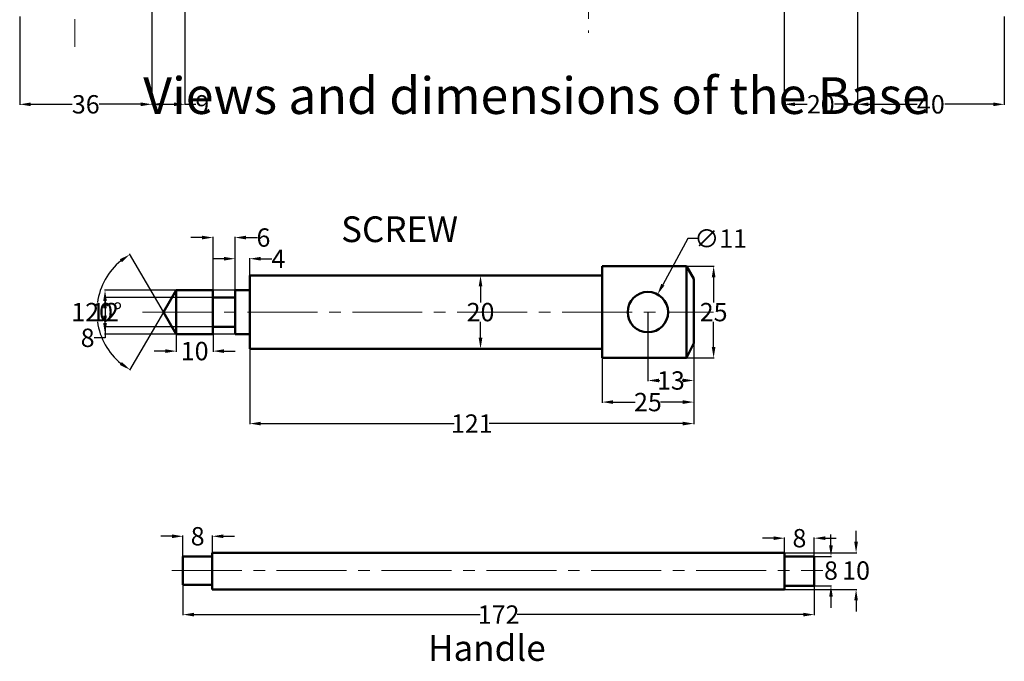
# Model space of a CAD drawing. Units: metres. Extents: x -2793 to -2360, y -31 to 491.
# Tile 1 of 4: x -2760 to -2492, y -31 to 144. Entities that reach past the tile are written whole.
import ezdxf

# ---------------------------------------------------------------- set-up
doc = ezdxf.new("R2010")
doc.units = ezdxf.units.M
doc.linetypes.add('CENTER2', pattern=[28.575, 19.05, -3.175, 3.175, -3.175])
for name, color, linetype, lineweight in [('M-CNTR', 9, 'CENTER2', 18), ('M-DIMS', 2, 'Continuous', 25), ('M-OUTL', 7, 'Continuous', 50), ('M-TEXT', 7, 'Continuous', 25)]:
    doc.layers.add(name, color=color, linetype=linetype, lineweight=lineweight)
doc.styles.get("Standard").update_dxf_attribs({"font": 'arial.ttf'})
doc.dimstyles.get("Standard").update_dxf_attribs({"dimtxt": 5, "dimasz": 3, "dimexe": 0.18, "dimexo": 0.0625, "dimgap": 0.09, "dimtad": 0, "dimtih": 1, "dimtoh": 1, "dimdec": 0, "dimzin": 0, "dimdsep": 46, "dimtxsty": 'Standard', "dimcen": 0.09, "dimclrd": 254, "dimclre": 254, "dimadec": 0, "dimazin": 0, "dimtfac": 1, "dimtdec": 0, "dimtofl": 0, "dimtmove": 0, "dimatfit": 3, "dimfxl": 1, "dimtolj": 1, "dimtzin": 0, "dimarcsym": 0})

# ---------------------------------------------------------------- blocks, each defined once
blk = doc.blocks.new('*D33')
at = {"layer": 'Defpoints', "color": 0, "transparency": 16777216}
for p in [(-2543.38, -1.94), (-2543.38, -9.94), (-2538.83, -9.94)]:
    blk.add_point(p, dxfattribs=at)
at = {"layer": 'M-DIMS', "color": 0, "lineweight": -2, "transparency": 16777216}
for p, q in [((-2538.83, 1.06), (-2538.83, 4.06)), ((-2543.32, -1.94), (-2538.65, -1.94)), ((-2543.32, -9.94), (-2538.65, -9.94)), ((-2538.83, -12.94), (-2538.83, -15.94))]:
    blk.add_line(p, q, dxfattribs=at)
at = {"layer": 'M-DIMS', "color": 0, "transparency": 16777216}
for points in [[(-2539.33, 1.06), (-2538.33, 1.06), (-2538.83, -1.94)], [(-2539.33, -12.94), (-2538.33, -12.94), (-2538.83, -9.94)]]:
    blk.add_solid(points, dxfattribs=at)
at = {"layer": 'M-DIMS', "color": 0, "transparency": 16777216, "insert": (-2538.83, -5.8), "char_height": 5, "attachment_point": 5}
blk.add_mtext('\\A1;{\\fTimes New Roman|b0|i0|c0|p18;8}', dxfattribs=at)
blk = doc.blocks.new('*D34')
at = {"layer": 'Defpoints', "color": 0, "transparency": 16777216}
for p in [(-2707.38, 3.55), (-2715.38, -1.94), (-2707.38, -1.94)]:
    blk.add_point(p, dxfattribs=at)
at = {"layer": 'M-DIMS', "color": 0, "lineweight": -2, "transparency": 16777216}
for p, q in [((-2718.38, 3.55), (-2721.38, 3.55)), ((-2715.38, -1.88), (-2715.38, 3.73)), ((-2707.38, -1.88), (-2707.38, 3.73)), ((-2704.38, 3.55), (-2701.38, 3.55))]:
    blk.add_line(p, q, dxfattribs=at)
at = {"layer": 'M-DIMS', "color": 0, "transparency": 16777216}
for points in [[(-2718.38, 4.05), (-2718.38, 3.05), (-2715.38, 3.55)], [(-2704.38, 4.05), (-2704.38, 3.05), (-2707.38, 3.55)]]:
    blk.add_solid(points, dxfattribs=at)
at = {"layer": 'M-DIMS', "color": 0, "transparency": 16777216, "insert": (-2711.38, 3.55), "char_height": 5, "attachment_point": 5}
blk.add_mtext('\\A1;{\\fTimes New Roman|b0|i0|c0|p18;8}', dxfattribs=at)
blk = doc.blocks.new('*D35')
at = {"layer": 'Defpoints', "color": 0, "transparency": 16777216}
for p in [(-2551.48, 3.03), (-2551.48, -1.94), (-2543.38, -1.94)]:
    blk.add_point(p, dxfattribs=at)
at = {"layer": 'M-DIMS', "color": 0, "lineweight": -2, "transparency": 16777216}
for p, q in [((-2554.48, 3.03), (-2557.48, 3.03)), ((-2551.48, -1.88), (-2551.48, 3.21)), ((-2543.38, -1.88), (-2543.38, 3.21)), ((-2540.38, 3.03), (-2537.38, 3.03))]:
    blk.add_line(p, q, dxfattribs=at)
at = {"layer": 'M-DIMS', "color": 0, "transparency": 16777216}
for points in [[(-2554.48, 3.53), (-2554.48, 2.53), (-2551.48, 3.03)], [(-2540.38, 3.53), (-2540.38, 2.53), (-2543.38, 3.03)]]:
    blk.add_solid(points, dxfattribs=at)
at = {"layer": 'M-DIMS', "color": 0, "transparency": 16777216, "insert": (-2547.43, 3.03), "char_height": 5, "attachment_point": 5}
blk.add_mtext('\\A1;{\\fTimes New Roman|b0|i0|c0|p18;8}', dxfattribs=at)
blk = doc.blocks.new('*D36')
at = {"layer": 'Defpoints', "color": 0, "transparency": 16777216}
for p in [(-2715.38, -9.66), (-2543.38, -9.94), (-2715.38, -17.79)]:
    blk.add_point(p, dxfattribs=at)
at = {"layer": 'M-DIMS', "color": 0, "lineweight": -2, "transparency": 16777216}
for p, q in [((-2715.38, -9.73), (-2715.38, -17.97)), ((-2543.38, -10), (-2543.38, -17.97)), ((-2712.38, -17.79), (-2634.43, -17.79)), ((-2546.38, -17.79), (-2624.34, -17.79))]:
    blk.add_line(p, q, dxfattribs=at)
at = {"layer": 'M-DIMS', "color": 0, "transparency": 16777216}
for points in [[(-2712.38, -17.29), (-2712.38, -18.29), (-2715.38, -17.79)], [(-2546.38, -17.29), (-2546.38, -18.29), (-2543.38, -17.79)]]:
    blk.add_solid(points, dxfattribs=at)
at = {"layer": 'M-DIMS', "color": 0, "transparency": 16777216, "insert": (-2629.38, -17.79), "char_height": 5, "attachment_point": 5}
blk.add_mtext('\\A1;{\\fTimes New Roman|b0|i0|c0|p18;172}', dxfattribs=at)
blk = doc.blocks.new('*D37')
at = {"layer": 'Defpoints', "color": 0, "transparency": 16777216}
for p in [(-2551.48, -0.94), (-2551.48, -10.94), (-2531.99, -10.94)]:
    blk.add_point(p, dxfattribs=at)
at = {"layer": 'M-DIMS', "color": 0, "lineweight": -2, "transparency": 16777216}
for p, q in [((-2531.99, 2.06), (-2531.99, 5.06)), ((-2551.42, -0.94), (-2531.81, -0.94)), ((-2551.42, -10.94), (-2531.81, -10.94)), ((-2531.99, -13.94), (-2531.99, -16.94))]:
    blk.add_line(p, q, dxfattribs=at)
at = {"layer": 'M-DIMS', "color": 0, "transparency": 16777216}
for points in [[(-2532.49, 2.06), (-2531.49, 2.06), (-2531.99, -0.94)], [(-2532.49, -13.94), (-2531.49, -13.94), (-2531.99, -10.94)]]:
    blk.add_solid(points, dxfattribs=at)
at = {"layer": 'M-DIMS', "color": 0, "transparency": 16777216, "insert": (-2531.99, -5.79), "char_height": 5, "attachment_point": 5}
blk.add_mtext('\\A1;{\\fTimes New Roman|b0|i0|c0|p18;10}', dxfattribs=at)
blk = doc.blocks.new('*D38')
at = {"layer": 'Defpoints', "color": 0, "transparency": 16777216}
for p in [(-2697.2, 54.62), (-2576.2, 56.14), (-2576.2, 34.25)]:
    blk.add_point(p, dxfattribs=at)
at = {"layer": 'M-DIMS', "color": 0, "lineweight": -2, "transparency": 16777216}
for p, q in [((-2697.2, 54.56), (-2697.2, 34.07)), ((-2576.2, 56.08), (-2576.2, 34.07)), ((-2694.2, 34.25), (-2641.45, 34.25)), ((-2579.2, 34.25), (-2631.96, 34.25))]:
    blk.add_line(p, q, dxfattribs=at)
at = {"layer": 'M-DIMS', "color": 0, "transparency": 16777216}
for points in [[(-2694.2, 34.75), (-2694.2, 33.75), (-2697.2, 34.25)], [(-2579.2, 34.75), (-2579.2, 33.75), (-2576.2, 34.25)]]:
    blk.add_solid(points, dxfattribs=at)
at = {"layer": 'M-DIMS', "color": 0, "transparency": 16777216, "insert": (-2636.7, 34.25), "char_height": 5, "attachment_point": 5}
blk.add_mtext('\\A1;{\\fTimes New Roman|b0|i0|c0|p18;121}', dxfattribs=at)
blk = doc.blocks.new('*D39')
at = {"layer": 'Defpoints', "color": 0, "transparency": 16777216}
for p in [(-2630.64, 74.62), (-2634.31, 54.62), (-2630.64, 54.62)]:
    blk.add_point(p, dxfattribs=at)
at = {"layer": 'M-DIMS', "color": 0, "lineweight": -2, "transparency": 16777216}
for p, q in [((-2630.71, 74.62), (-2634.49, 74.62)), ((-2634.31, 71.62), (-2634.31, 67.26)), ((-2634.31, 57.62), (-2634.31, 61.99)), ((-2630.71, 54.62), (-2634.49, 54.62))]:
    blk.add_line(p, q, dxfattribs=at)
at = {"layer": 'M-DIMS', "color": 0, "transparency": 16777216}
for points in [[(-2634.81, 71.62), (-2633.81, 71.62), (-2634.31, 74.62)], [(-2634.81, 57.62), (-2633.81, 57.62), (-2634.31, 54.62)]]:
    blk.add_solid(points, dxfattribs=at)
at = {"layer": 'M-DIMS', "color": 0, "transparency": 16777216, "insert": (-2634.31, 64.62), "char_height": 5, "attachment_point": 5}
blk.add_mtext('\\A1;{\\fTimes New Roman|b0|i0|c0|p18;20}', dxfattribs=at)
blk = doc.blocks.new('*D40')
at = {"layer": 'Defpoints', "color": 0, "transparency": 16777216}
for p in [(-2601.2, 52.12), (-2576.2, 52.12), (-2576.2, 40.11)]:
    blk.add_point(p, dxfattribs=at)
at = {"layer": 'M-DIMS', "color": 0, "lineweight": -2, "transparency": 16777216}
for p, q in [((-2601.2, 52.06), (-2601.2, 39.93)), ((-2576.2, 52.06), (-2576.2, 39.93)), ((-2598.2, 40.11), (-2592.16, 40.11)), ((-2579.2, 40.11), (-2585.25, 40.11))]:
    blk.add_line(p, q, dxfattribs=at)
at = {"layer": 'M-DIMS', "color": 0, "transparency": 16777216}
for points in [[(-2598.2, 40.61), (-2598.2, 39.61), (-2601.2, 40.11)], [(-2579.2, 40.61), (-2579.2, 39.61), (-2576.2, 40.11)]]:
    blk.add_solid(points, dxfattribs=at)
at = {"layer": 'M-DIMS', "color": 0, "transparency": 16777216, "insert": (-2588.7, 40.11), "char_height": 5, "attachment_point": 5}
blk.add_mtext('\\A1;{\\fTimes New Roman|b0|i0|c0|p18;25}', dxfattribs=at)
blk = doc.blocks.new('*D41')
at = {"layer": 'Defpoints', "color": 0, "transparency": 16777216}
for p in [(-2588.7, 64.62), (-2576.2, 64.62), (-2576.2, 45.99)]:
    blk.add_point(p, dxfattribs=at)
at = {"layer": 'M-DIMS', "color": 0, "lineweight": -2, "transparency": 16777216}
for p, q in [((-2588.7, 64.56), (-2588.7, 45.81)), ((-2576.2, 64.56), (-2576.2, 45.81)), ((-2585.7, 45.99), (-2585.5, 45.99)), ((-2579.2, 45.99), (-2579.41, 45.99))]:
    blk.add_line(p, q, dxfattribs=at)
at = {"layer": 'M-DIMS', "color": 0, "transparency": 16777216}
for points in [[(-2585.7, 46.49), (-2585.7, 45.49), (-2588.7, 45.99)], [(-2579.2, 46.49), (-2579.2, 45.49), (-2576.2, 45.99)]]:
    blk.add_solid(points, dxfattribs=at)
at = {"layer": 'M-DIMS', "color": 0, "transparency": 16777216, "insert": (-2582.45, 45.99), "char_height": 5, "attachment_point": 5}
blk.add_mtext('\\A1;{\\fTimes New Roman|b0|i0|c0|p18;13}', dxfattribs=at)
blk = doc.blocks.new('*D42')
at = {"layer": 'Defpoints', "color": 0, "transparency": 16777216}
for p in [(-2578.2, 77.12), (-2578.2, 52.12), (-2570.8, 52.12)]:
    blk.add_point(p, dxfattribs=at)
at = {"layer": 'M-DIMS', "color": 0, "lineweight": -2, "transparency": 16777216}
for p, q in [((-2578.14, 77.12), (-2570.62, 77.12)), ((-2570.8, 74.12), (-2570.8, 67.26)), ((-2570.8, 55.12), (-2570.8, 61.99)), ((-2578.14, 52.12), (-2570.62, 52.12))]:
    blk.add_line(p, q, dxfattribs=at)
at = {"layer": 'M-DIMS', "color": 0, "transparency": 16777216}
for points in [[(-2571.3, 74.12), (-2570.3, 74.12), (-2570.8, 77.12)], [(-2571.3, 55.12), (-2570.3, 55.12), (-2570.8, 52.12)]]:
    blk.add_solid(points, dxfattribs=at)
at = {"layer": 'M-DIMS', "color": 0, "transparency": 16777216, "insert": (-2570.8, 64.62), "char_height": 5, "attachment_point": 5}
blk.add_mtext('\\A1;{\\fTimes New Roman|b0|i0|c0|p18;25}', dxfattribs=at)
blk = doc.blocks.new('*D43')
at = {"layer": 'Defpoints', "color": 0, "transparency": 16777216}
for p in [(-2586.08, 69.45), (-2591.33, 59.79)]:
    blk.add_point(p, dxfattribs=at)
at = {"layer": 'M-DIMS', "color": 0, "lineweight": -2, "transparency": 16777216}
for p, q in [((-2577.81, 84.65), (-2584.64, 72.09)), ((-2574.77, 84.65), (-2577.81, 84.65)), ((-2588.79, 64.62), (-2588.61, 64.62)), ((-2588.7, 64.53), (-2588.7, 64.71))]:
    blk.add_line(p, q, dxfattribs=at)
at = {"layer": 'M-DIMS', "color": 0, "transparency": 16777216}
blk.add_solid([(-2585.08, 72.33), (-2584.2, 71.85), (-2586.08, 69.45)], dxfattribs=at)
at = {"layer": 'M-DIMS', "color": 0, "transparency": 16777216, "insert": (-2568.9, 84.65), "char_height": 5, "attachment_point": 5}
blk.add_mtext('\\A1;{\\fTimes New Roman|b0|i0|c0|p18;∅11}', dxfattribs=at)
blk = doc.blocks.new('*D44')
at = {"layer": 'Defpoints', "color": 0, "transparency": 16777216}
for p in [(-2697.2, 79.16), (-2701.2, 70.62), (-2697.2, 70.62)]:
    blk.add_point(p, dxfattribs=at)
at = {"layer": 'M-DIMS', "color": 0, "lineweight": -2, "transparency": 16777216}
for p, q in [((-2704.2, 79.16), (-2707.2, 79.16)), ((-2701.2, 70.68), (-2701.2, 79.34)), ((-2697.2, 70.68), (-2697.2, 79.34)), ((-2694.2, 79.16), (-2691.14, 79.16))]:
    blk.add_line(p, q, dxfattribs=at)
at = {"layer": 'M-DIMS', "color": 0, "transparency": 16777216}
for points in [[(-2704.2, 79.66), (-2704.2, 78.66), (-2701.2, 79.16)], [(-2694.2, 79.66), (-2694.2, 78.66), (-2697.2, 79.16)]]:
    blk.add_solid(points, dxfattribs=at)
at = {"layer": 'M-DIMS', "color": 0, "transparency": 16777216, "insert": (-2689.39, 79.16), "char_height": 5, "attachment_point": 5}
blk.add_mtext('\\A1;{\\fTimes New Roman|b0|i0|c0|p18;4}', dxfattribs=at)
blk = doc.blocks.new('*D45')
at = {"layer": 'Defpoints', "color": 0, "transparency": 16777216}
for p in [(-2701.2, 84.93), (-2707.2, 68.62), (-2701.2, 68.62)]:
    blk.add_point(p, dxfattribs=at)
at = {"layer": 'M-DIMS', "color": 0, "lineweight": -2, "transparency": 16777216}
for p, q in [((-2710.2, 84.93), (-2713.2, 84.93)), ((-2707.2, 68.68), (-2707.2, 85.11)), ((-2701.2, 68.68), (-2701.2, 85.11)), ((-2698.2, 84.93), (-2695.1, 84.93))]:
    blk.add_line(p, q, dxfattribs=at)
at = {"layer": 'M-DIMS', "color": 0, "transparency": 16777216}
for points in [[(-2710.2, 85.43), (-2710.2, 84.43), (-2707.2, 84.93)], [(-2698.2, 85.43), (-2698.2, 84.43), (-2701.2, 84.93)]]:
    blk.add_solid(points, dxfattribs=at)
at = {"layer": 'M-DIMS', "color": 0, "transparency": 16777216, "insert": (-2693.46, 84.93), "char_height": 5, "attachment_point": 5}
blk.add_mtext('\\A1;{\\fTimes New Roman|b0|i0|c0|p18;6}', dxfattribs=at)
blk = doc.blocks.new('*D46')
at = {"layer": 'Defpoints', "color": 0, "transparency": 16777216}
for p in [(-2717.2, 58.62), (-2707.2, 58.62), (-2707.2, 54)]:
    blk.add_point(p, dxfattribs=at)
at = {"layer": 'M-DIMS', "color": 0, "lineweight": -2, "transparency": 16777216}
for p, q in [((-2717.2, 58.56), (-2717.2, 53.82)), ((-2707.2, 58.56), (-2707.2, 53.82)), ((-2720.2, 54), (-2723.2, 54)), ((-2704.2, 54), (-2701.2, 54))]:
    blk.add_line(p, q, dxfattribs=at)
at = {"layer": 'M-DIMS', "color": 0, "transparency": 16777216}
for points in [[(-2720.2, 54.5), (-2720.2, 53.5), (-2717.2, 54)], [(-2704.2, 54.5), (-2704.2, 53.5), (-2707.2, 54)]]:
    blk.add_solid(points, dxfattribs=at)
at = {"layer": 'M-DIMS', "color": 0, "transparency": 16777216, "insert": (-2712.2, 54), "char_height": 5, "attachment_point": 5}
blk.add_mtext('\\A1;{\\fTimes New Roman|b0|i0|c0|p18;10}', dxfattribs=at)
blk = doc.blocks.new('*D47')
at = {"layer": 'Defpoints', "color": 0, "transparency": 16777216}
for p in [(-2737.79, 70.82), (-2717.2, 70.62), (-2720.7, 64.62), (-2720.7, 64.62), (-2717.2, 58.62)]:
    blk.add_point(p, dxfattribs=at)
at = {"layer": 'M-DIMS', "color": 0, "lineweight": -2, "transparency": 16777216}
for p, q in [((-2720.73, 64.68), (-2729.93, 80.48)), ((-2720.73, 64.57), (-2729.93, 48.76))]:
    blk.add_line(p, q, dxfattribs=at)
for start, end in [(129.677, 171.6699), (188.3301, 230.323)]:
    blk.add_arc((-2720.7, 64.62), 18.18, start, end, dxfattribs=at)
at = {"layer": 'M-DIMS', "color": 0, "transparency": 16777216}
for points in [[(-2732.59, 79.02), (-2732.02, 78.2), (-2729.84, 80.33)], [(-2732.02, 51.04), (-2732.59, 50.22), (-2729.84, 48.91)]]:
    blk.add_solid(points, dxfattribs=at)
at = {"layer": 'M-DIMS', "color": 0, "transparency": 16777216, "insert": (-2738.87, 64.62), "char_height": 5, "attachment_point": 5}
blk.add_mtext('\\A1;{\\fTimes New Roman|b0|i0|c0|p18;120°}', dxfattribs=at)
blk = doc.blocks.new('*D56')
at = {"layer": 'Defpoints', "color": 0, "transparency": 16777216}
for p in [(-2723.87, 168.18), (-2759.87, 145.18), (-2723.87, 121.23)]:
    blk.add_point(p, dxfattribs=at)
at = {"layer": 'M-DIMS', "color": 254, "lineweight": -2, "transparency": 16777216}
for p, q in [((-2723.87, 168.11), (-2723.87, 121.05)), ((-2759.87, 145.11), (-2759.87, 121.05)), ((-2756.87, 121.23), (-2745.54, 121.23)), ((-2726.87, 121.23), (-2738.2, 121.23))]:
    blk.add_line(p, q, dxfattribs=at)
at = {"layer": 'M-DIMS', "color": 254, "transparency": 16777216}
for points in [[(-2756.87, 121.73), (-2756.87, 120.73), (-2759.87, 121.23)], [(-2726.87, 121.73), (-2726.87, 120.73), (-2723.87, 121.23)]]:
    blk.add_solid(points, dxfattribs=at)
at = {"layer": 'M-DIMS', "color": 0, "transparency": 16777216, "insert": (-2741.87, 121.23), "char_height": 5, "attachment_point": 5}
blk.add_mtext('\\A1;36', dxfattribs=at)
blk = doc.blocks.new('*D57')
at = {"layer": 'Defpoints', "color": 0, "transparency": 16777216}
for p in [(-2723.87, 168.18), (-2714.87, 168.18), (-2714.87, 121.23)]:
    blk.add_point(p, dxfattribs=at)
at = {"layer": 'M-DIMS', "color": 254, "lineweight": -2, "transparency": 16777216}
for p, q in [((-2723.87, 168.11), (-2723.87, 121.05)), ((-2714.87, 168.11), (-2714.87, 121.05)), ((-2720.87, 121.23), (-2717.87, 121.23)), ((-2714.87, 121.23), (-2711.87, 121.23))]:
    blk.add_line(p, q, dxfattribs=at)
at = {"layer": 'M-DIMS', "color": 254, "transparency": 16777216}
for points in [[(-2720.87, 121.73), (-2720.87, 120.73), (-2723.87, 121.23)], [(-2717.87, 121.73), (-2717.87, 120.73), (-2714.87, 121.23)]]:
    blk.add_solid(points, dxfattribs=at)
at = {"layer": 'M-DIMS', "color": 0, "transparency": 16777216, "insert": (-2710.13, 121.23), "char_height": 5, "attachment_point": 5}
blk.add_mtext('\\A1;9', dxfattribs=at)
blk = doc.blocks.new('*D58')
at = {"layer": 'Defpoints', "color": 0, "transparency": 16777216}
for p in [(-2531.61, 168.18), (-2551.61, 165.18), (-2531.61, 121.23)]:
    blk.add_point(p, dxfattribs=at)
at = {"layer": 'M-DIMS', "color": 254, "lineweight": -2, "transparency": 16777216}
for p, q in [((-2531.61, 168.11), (-2531.61, 121.05)), ((-2551.61, 165.11), (-2551.61, 121.05)), ((-2548.61, 121.23), (-2545.31, 121.23)), ((-2534.61, 121.23), (-2537.9, 121.23))]:
    blk.add_line(p, q, dxfattribs=at)
at = {"layer": 'M-DIMS', "color": 254, "transparency": 16777216}
for points in [[(-2548.61, 121.73), (-2548.61, 120.73), (-2551.61, 121.23)], [(-2534.61, 121.73), (-2534.61, 120.73), (-2531.61, 121.23)]]:
    blk.add_solid(points, dxfattribs=at)
at = {"layer": 'M-DIMS', "color": 0, "transparency": 16777216, "insert": (-2541.61, 121.23), "char_height": 5, "attachment_point": 5}
blk.add_mtext('\\A1;20', dxfattribs=at)
blk = doc.blocks.new('*D59')
at = {"layer": 'Defpoints', "color": 0, "transparency": 16777216}
for p in [(-2531.61, 168.18), (-2491.61, 145.18), (-2491.61, 121.23)]:
    blk.add_point(p, dxfattribs=at)
at = {"layer": 'M-DIMS', "color": 254, "lineweight": -2, "transparency": 16777216}
for p, q in [((-2531.61, 168.11), (-2531.61, 121.05)), ((-2491.61, 145.11), (-2491.61, 121.05)), ((-2528.61, 121.23), (-2515.37, 121.23)), ((-2494.61, 121.23), (-2507.84, 121.23))]:
    blk.add_line(p, q, dxfattribs=at)
at = {"layer": 'M-DIMS', "color": 254, "transparency": 16777216}
for points in [[(-2528.61, 121.73), (-2528.61, 120.73), (-2531.61, 121.23)], [(-2494.61, 121.73), (-2494.61, 120.73), (-2491.61, 121.23)]]:
    blk.add_solid(points, dxfattribs=at)
at = {"layer": 'M-DIMS', "color": 0, "transparency": 16777216, "insert": (-2511.61, 121.23), "char_height": 5, "attachment_point": 5}
blk.add_mtext('\\A1;40', dxfattribs=at)
blk = doc.blocks.new('*D63')
at = {"layer": 'Defpoints', "color": 0, "transparency": 16777216}
for p in [(-2717.2, 70.62), (-2736.62, 58.62), (-2717.2, 58.62)]:
    blk.add_point(p, dxfattribs=at)
at = {"layer": 'M-DIMS', "color": 254, "lineweight": -2, "transparency": 16777216}
for p, q in [((-2717.27, 70.62), (-2736.8, 70.62)), ((-2736.62, 67.62), (-2736.62, 67.22)), ((-2736.62, 61.62), (-2736.62, 62.02)), ((-2717.27, 58.62), (-2736.8, 58.62))]:
    blk.add_line(p, q, dxfattribs=at)
at = {"layer": 'M-DIMS', "color": 254, "transparency": 16777216}
for points in [[(-2737.12, 67.62), (-2736.12, 67.62), (-2736.62, 70.62)], [(-2737.12, 61.62), (-2736.12, 61.62), (-2736.62, 58.62)]]:
    blk.add_solid(points, dxfattribs=at)
at = {"layer": 'M-DIMS', "color": 0, "transparency": 16777216, "insert": (-2736.62, 64.62), "char_height": 5, "attachment_point": 5}
blk.add_mtext('\\A1;12', dxfattribs=at)
blk = doc.blocks.new('*D64')
at = {"layer": 'Defpoints', "color": 0, "transparency": 16777216}
for p in [(-2707.2, 68.62), (-2736.62, 60.62), (-2707.2, 60.62)]:
    blk.add_point(p, dxfattribs=at)
at = {"layer": 'M-DIMS', "color": 254, "lineweight": -2, "transparency": 16777216}
for p, q in [((-2707.27, 68.62), (-2736.8, 68.62)), ((-2736.62, 65.62), (-2736.62, 63.62)), ((-2707.27, 60.62), (-2736.8, 60.62)), ((-2736.62, 60.62), (-2736.62, 57.62)), ((-2736.62, 57.62), (-2739.62, 57.62))]:
    blk.add_line(p, q, dxfattribs=at)
at = {"layer": 'M-DIMS', "color": 254, "transparency": 16777216}
for points in [[(-2737.12, 65.62), (-2736.12, 65.62), (-2736.62, 68.62)], [(-2737.12, 63.62), (-2736.12, 63.62), (-2736.62, 60.62)]]:
    blk.add_solid(points, dxfattribs=at)
at = {"layer": 'M-DIMS', "color": 0, "transparency": 16777216, "insert": (-2741.36, 57.62), "char_height": 5, "attachment_point": 5}
blk.add_mtext('\\A1;8', dxfattribs=at)
blk = doc.blocks.new('*D65')
at = {"layer": 'Defpoints', "color": 0, "transparency": 16777216}
for p in [(-2697.2, 70.62), (-2736.62, 58.62), (-2697.2, 58.62)]:
    blk.add_point(p, dxfattribs=at)
at = {"layer": 'M-DIMS', "color": 254, "lineweight": -2, "transparency": 16777216}
for p, q in [((-2697.27, 70.62), (-2736.8, 70.62)), ((-2736.62, 67.62), (-2736.62, 67.22)), ((-2736.62, 61.62), (-2736.62, 62.02)), ((-2697.27, 58.62), (-2736.8, 58.62))]:
    blk.add_line(p, q, dxfattribs=at)
at = {"layer": 'M-DIMS', "color": 254, "transparency": 16777216}
for points in [[(-2737.12, 67.62), (-2736.12, 67.62), (-2736.62, 70.62)], [(-2737.12, 61.62), (-2736.12, 61.62), (-2736.62, 58.62)]]:
    blk.add_solid(points, dxfattribs=at)
at = {"layer": 'M-DIMS', "color": 0, "transparency": 16777216, "insert": (-2736.62, 64.62), "char_height": 5, "attachment_point": 5}
blk.add_mtext('\\A1;12', dxfattribs=at)

msp = doc.modelspace()

# ---------------------------------------------------------------- linework, layer by layer
at = {"layer": 'M-CNTR'}
for p, q in [((-2744.868, 172.975), (-2744.868, 136.879)), ((-2604.868, 169.913), (-2604.868, 140.718)), ((-2726.374, 64.622), (-2570.796, 64.622)), ((-2718.429, -5.802), (-2541.084, -5.802))]:
    msp.add_line(p, q, dxfattribs=at)
at = {"layer": 'M-OUTL'}
for p, q in [((-2578.205, 77.122), (-2601.205, 77.122)), ((-2601.205, 52.122), (-2601.205, 77.122)), ((-2578.205, 52.122), (-2578.205, 77.122)), ((-2578.205, 77.122), (-2576.205, 73.679)), ((-2697.205, 74.622), (-2697.205, 54.622)), ((-2697.205, 74.622), (-2601.205, 74.622)), ((-2576.205, 56.143), (-2576.205, 73.679)), ((-2576.205, 73.679), (-2576.205, 56.595)), ((-2720.698, 64.622), (-2717.205, 70.622)), ((-2717.205, 70.622), (-2717.205, 58.622)), ((-2717.205, 70.622), (-2707.205, 70.622)), ((-2707.205, 70.622), (-2707.205, 58.622)), ((-2701.205, 70.622), (-2701.205, 58.622)), ((-2701.205, 70.622), (-2697.205, 70.622)), ((-2707.205, 68.622), (-2701.205, 68.622)), ((-2717.205, 58.622), (-2720.698, 64.622)), ((-2707.205, 60.622), (-2701.205, 60.622)), ((-2717.205, 58.622), (-2707.205, 58.622)), ((-2701.205, 58.622), (-2697.205, 58.622)), ((-2697.205, 54.622), (-2601.205, 54.622)), ((-2576.205, 56.143), (-2578.205, 52.122)), ((-2601.205, 52.122), (-2578.205, 52.122)), ((-2715.384, -1.941), (-2715.384, -9.663)), ((-2707.384, -1.941), (-2715.384, -1.941)), ((-2551.479, -0.941), (-2707.384, -0.941)), ((-2707.384, -0.941), (-2707.384, -10.941)), ((-2551.479, -10.941), (-2551.479, -0.941)), ((-2543.384, -1.941), (-2551.479, -1.941)), ((-2543.384, -9.941), (-2543.384, -1.941)), ((-2715.384, -9.663), (-2707.384, -9.663)), ((-2551.479, -9.941), (-2543.384, -9.941)), ((-2707.384, -10.941), (-2551.479, -10.941))]:
    msp.add_line(p, q, dxfattribs=at)
msp.add_circle((-2588.705, 64.622), 5.5, dxfattribs=at)

# ---------------------------------------------------------------- texts
at = {"layer": 'M-TEXT', "attachment_point": 1}
for s, width, insert, char_height in [('{\\fTimes New Roman|b0|i0|c0|p18;Views and dimensions of the Base}', 226.31476, (-2726.218, 128.599), 10), ('{\\fTimes New Roman|b0|i0|c0|p18;SCREW}', 66.81004, (-2672.301, 90.698), 7), ('{\\fTimes New Roman|b0|i0|c0|p18;Handle}', 80.88995, (-2648.631, -23.39), 7)]:
    msp.add_mtext_dynamic_manual_height_columns(s, width=width, gutter_width=12.5, heights=[0], dxfattribs=dict(at, insert=insert, char_height=char_height))

# ---------------------------------------------------------------- dimensions: what is measured, and where the dimension line sits
at = {"layer": 'M-DIMS'}
for base, p1, p2, picture, middle in [((-2723.868, 121.229), (-2759.868, 145.175), (-2723.868, 168.175), '*D56', (-2741.868, 121.229)), ((-2714.868, 121.229), (-2723.868, 168.175), (-2714.868, 168.175), '*D57', (-2710.134, 121.229)), ((-2531.605, 121.229), (-2551.605, 165.175), (-2531.605, 168.175), '*D58', (-2541.605, 121.229)), ((-2491.605, 121.229), (-2531.605, 168.175), (-2491.605, 145.175), '*D59', (-2511.605, 121.229))]:
    dim = msp.add_linear_dim(base=base, p1=p1, p2=p2, dimstyle='Standard', override={"dimdec": 0, "dimlfac": 1, "dimrnd": 0, "dimzin": 0, "dimdsep": 46, "dimlunit": 2}, dxfattribs=at)
    dim.commit()
    dim.dimension.update_dxf_attribs({"geometry": picture, "text_midpoint": middle})
for base, p1, p2, text, picture, middle in [((-2701.205, 84.927), (-2707.205, 68.622), (-2701.205, 68.622), '{\\fTimes New Roman|b0|i0|c0|p18;6}', '*D45', (-2693.464, 84.927)), ((-2697.205, 79.162), (-2701.205, 70.622), (-2697.205, 70.622), '{\\fTimes New Roman|b0|i0|c0|p18;<>}', '*D44', (-2689.386, 79.162)), ((-2576.204782659, 45.993769251), (-2588.704782659, 64.621782455), (-2576.204782659, 64.621782455), '{\\fTimes New Roman|b0|i0|c0|p18;<>}', '*D41', (-2582.454782659, 45.993769251)), ((-2576.205, 34.252), (-2697.205, 54.622), (-2576.205, 56.143), '{\\fTimes New Roman|b0|i0|c0|p18;<>}', '*D38', (-2636.705, 34.252)), ((-2576.205, 40.11), (-2601.205, 52.122), (-2576.205, 52.122), '{\\fTimes New Roman|b0|i0|c0|p18;<>}', '*D40', (-2588.705, 40.11)), ((-2707.384, 3.554), (-2715.384, -1.941), (-2707.384, -1.941), '{\\fTimes New Roman|b0|i0|c0|p18;<>}', '*D34', (-2711.384, 3.554)), ((-2551.479, 3.032), (-2543.384, -1.941), (-2551.479, -1.941), '{\\fTimes New Roman|b0|i0|c0|p18;<>}', '*D35', (-2547.432, 3.032))]:
    dim = msp.add_linear_dim(base=base, p1=p1, p2=p2, text=text, dimstyle='Standard', override={"dimclrd": 0, "dimclre": 0, "dimclrt": 0}, dxfattribs=at)
    dim.commit()
    dim.dimension.update_dxf_attribs({"geometry": picture, "text_midpoint": middle, "dimtype": 160})
dim = msp.add_diameter_dim_2p(p1=(-2591.333, 59.79), p2=(-2586.077, 69.453), text='{\\fTimes New Roman|b0|i0|c0|p18;<>}', dimstyle='Standard', override={"dimclrd": 0, "dimclre": 0, "dimclrt": 0}, dxfattribs=at)
dim.commit()
dim.dimension.update_dxf_attribs({"geometry": '*D43', "text_midpoint": (-2568.904, 84.649), "dimtype": 163})
dim = msp.add_angular_dim_2l(base=(-2737.785, 70.817), line1=((-2720.698, 64.622), (-2717.205, 70.622)), line2=((-2717.205, 58.622), (-2720.698, 64.622)), text='{\\fTimes New Roman|b0|i0|c0|p18;<>}', dimstyle='Standard', override={"dimclrd": 0, "dimclre": 0, "dimclrt": 0}, dxfattribs=at)
dim.commit()
dim.dimension.update_dxf_attribs({"geometry": '*D47', "text_midpoint": (-2738.874, 64.622)})
for base, p1, p2, picture, middle in [((-2570.796, 52.122), (-2578.205, 77.122), (-2578.205, 52.122), '*D42', (-2570.796, 64.622)), ((-2634.311, 54.622), (-2630.644, 74.622), (-2630.644, 54.622), '*D39', (-2634.311, 64.622))]:
    dim = msp.add_linear_dim(base=base, p1=p1, p2=p2, angle=90, text='{\\fTimes New Roman|b0|i0|c0|p18;<>}', dimstyle='Standard', override={"dimclrd": 0, "dimclre": 0, "dimclrt": 0}, dxfattribs=at)
    dim.commit()
    dim.dimension.update_dxf_attribs({"geometry": picture, "text_midpoint": middle})
for base, p1, p2, picture, middle in [((-2736.624, 58.622), (-2717.205, 70.622), (-2717.205, 58.622), '*D63', (-2736.624, 64.622)), ((-2736.624, 58.622), (-2697.205, 70.622), (-2697.205, 58.622), '*D65', (-2736.624, 64.622)), ((-2736.624, 60.622), (-2707.205, 68.622), (-2707.205, 60.622), '*D64', (-2741.361, 57.622))]:
    dim = msp.add_linear_dim(base=base, p1=p1, p2=p2, angle=90, dimstyle='Standard', override={"dimdec": 0, "dimlfac": 1, "dimrnd": 0, "dimzin": 0, "dimdsep": 46, "dimlunit": 2}, dxfattribs=at)
    dim.commit()
    dim.dimension.update_dxf_attribs({"geometry": picture, "text_midpoint": middle})
for base, p1, p2, picture, middle in [((-2707.205, 54.003), (-2717.205, 58.622), (-2707.205, 58.622), '*D46', (-2712.205, 54.003)), ((-2715.384, -17.789), (-2543.384, -9.941), (-2715.384, -9.663), '*D36', (-2629.384, -17.789))]:
    dim = msp.add_linear_dim(base=base, p1=p1, p2=p2, text='{\\fTimes New Roman|b0|i0|c0|p18;<>}', dimstyle='Standard', override={"dimclrd": 0, "dimclre": 0, "dimclrt": 0}, dxfattribs=at)
    dim.commit()
    dim.dimension.update_dxf_attribs({"geometry": picture, "text_midpoint": middle})
for base, p1, p2, picture, middle in [((-2531.985, -10.941), (-2551.479, -0.941), (-2551.479, -10.941), '*D37', (-2531.985, -5.789)), ((-2538.831, -9.941), (-2543.384, -1.941), (-2543.384, -9.941), '*D33', (-2538.831, -5.802))]:
    dim = msp.add_linear_dim(base=base, p1=p1, p2=p2, angle=90, text='{\\fTimes New Roman|b0|i0|c0|p18;<>}', dimstyle='Standard', override={"dimclrd": 0, "dimclre": 0, "dimclrt": 0}, dxfattribs=at)
    dim.commit()
    dim.dimension.update_dxf_attribs({"geometry": picture, "text_midpoint": middle, "dimtype": 160})

doc.saveas('drawing.dxf')
